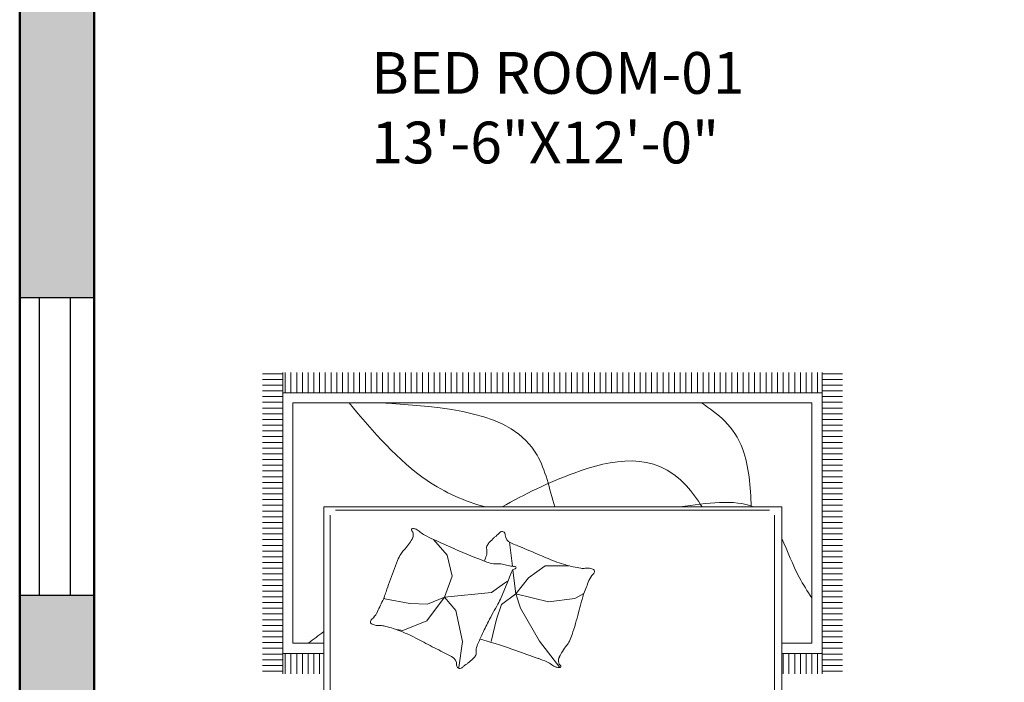
# Model space of a CAD drawing. Units: inches. Extents: x -7 to 1228, y -146 to 1091.
# Tile 4 of 88: x 60 to 179, y 112 to 193. Entities that reach past the tile are written whole.
import ezdxf

# ---------------------------------------------------------------- set-up
doc = ezdxf.new("R2010")
doc.units = ezdxf.units.IN
for name, color, linetype, lineweight in [('A-AREA-IDEN', 7, 'Continuous', 18), ('A-FURN', 8, 'Continuous', 18), ('A-GLAZ', 175, 'Continuous', 25), ('A-WALL', 7, 'Continuous', 50), ('A-WALL-PATT', 251, 'Continuous', 13)]:
    doc.layers.add(name, color=color, linetype=linetype, lineweight=lineweight)
doc.styles.add('DIM_FONT', font='SIMPLEX.shx', dxfattribs={"width": 0.8})
doc.styles.get("Standard").update_dxf_attribs({"font": 'arial.ttf'})

# ---------------------------------------------------------------- blocks, each defined once
blk = doc.blocks.new('A$C4F634EDD')
for p, q in [((0.5, 0.5295), (0.5, 2.6295)), ((2.3, 2.6295), (2.3, 0.5295)), ((0.5258, 2.121), (0.5258, 0.5617)), ((2.2716, 0.5617), (2.2716, 1.7136)), ((0.2586, 1.1753), (0.3386, 1.1753)), ((0.3386, 0), (0.3386, 1.1852)), ((0.3486, 1.1052), (0.3486, 1.1852)), ((0.3711, 1.1052), (0.3711, 1.1852)), ((0.3936, 1.1052), (0.3936, 1.1852)), ((0.4161, 1.1052), (0.4161, 1.1852)), ((0.4386, 1.1052), (0.4386, 1.1852)), ((0.4611, 1.1052), (0.4611, 1.1852)), ((0.4836, 1.1052), (0.4836, 1.1852)), ((1.031, 1.1612), (1.0448, 1.0581)), ((2.3061, 1.1052), (2.3061, 1.1852)), ((2.3286, 1.1052), (2.3286, 1.1852)), ((2.3511, 1.1052), (2.3511, 1.1852)), ((2.3736, 1.1052), (2.3736, 1.1852)), ((2.3961, 1.1052), (2.3961, 1.1852)), ((2.4186, 1.1052), (2.4186, 1.1852)), ((2.4411, 1.1052), (2.4411, 1.1852)), ((2.4588, 1.1852), (2.4588, 0)), ((2.4588, 1.1753), (2.5388, 1.1753)), ((0.2586, 1.1528), (0.3386, 1.1528)), ((0.2586, 1.1303), (0.3386, 1.1303)), ((1.4276, 1.1611), (1.3484, 1.0571)), ((2.4588, 1.1528), (2.5388, 1.1528)), ((2.4588, 1.1303), (2.5388, 1.1303)), ((0.2586, 1.1078), (0.3386, 1.1078)), ((0.2586, 1.0853), (0.3386, 1.0853)), ((0.3386, 1.1052), (0.5, 1.1052)), ((2.3, 1.1052), (2.4588, 1.1052)), ((2.4588, 1.1078), (2.5388, 1.1078)), ((2.4588, 1.0853), (2.5388, 1.0853)), ((0.2586, 1.0628), (0.3386, 1.0628)), ((0.3786, 1.0652), (0.5, 1.0652)), ((0.3786, 0.12), (0.3786, 1.0652)), ((1.0448, 1.0581), (1.019, 0.936)), ((1.1784, 0.9702), (1.1586, 1.0591)), ((1.3484, 1.0571), (1.2733, 0.9268)), ((2.3, 1.0652), (2.4188, 1.0652)), ((2.4188, 1.0652), (2.4188, 0.12)), ((2.4588, 1.0628), (2.5388, 1.0628)), ((0.2586, 1.0403), (0.3386, 1.0403)), ((0.2586, 1.0178), (0.3386, 1.0178)), ((0.8108, 1.0151), (0.7868, 1.0117)), ((0.9054, 0.9773), (0.8108, 1.0151)), ((2.4588, 1.0403), (2.5388, 1.0403)), ((2.4588, 1.0178), (2.5388, 1.0178)), ((0.2586, 0.9953), (0.3386, 0.9953)), ((0.2586, 0.9728), (0.3386, 0.9728)), ((0.9743, 0.8845), (0.9054, 0.9773)), ((1.1982, 0.9129), (1.1784, 0.9702)), ((2.4588, 0.9953), (2.5388, 0.9953)), ((2.4588, 0.9728), (2.5388, 0.9728)), ((0.2586, 0.9503), (0.3386, 0.9503)), ((1.019, 0.936), (0.9743, 0.8845)), ((2.4588, 0.9503), (2.5388, 0.9503)), ((0.2586, 0.9278), (0.3386, 0.9278)), ((0.2586, 0.9053), (0.3386, 0.9053)), ((0.7403, 0.8913), (0.737, 0.8849)), ((0.8384, 0.9085), (0.7403, 0.8913)), ((0.9072, 0.912), (0.8384, 0.9085)), ((0.9743, 0.8845), (0.9072, 0.912)), ((1.2555, 0.8715), (1.1982, 0.9129)), ((1.2733, 0.9268), (1.2555, 0.8715)), ((1.2555, 0.8715), (1.384, 0.9031)), ((1.384, 0.9031), (1.4868, 0.8892)), ((2.4588, 0.9278), (2.5388, 0.9278)), ((2.4588, 0.9053), (2.5388, 0.9053)), ((0.2586, 0.8828), (0.3386, 0.8828)), ((0.2586, 0.8603), (0.3386, 0.8603)), ((0.9743, 0.8845), (1.0052, 0.802)), ((0.9743, 0.8845), (1.16, 0.8656)), ((1.16, 0.8656), (1.2099, 0.8295)), ((1.1973, 0.8853), (1.2203, 0.829)), ((1.2555, 0.8715), (1.2437, 0.7773)), ((1.2555, 0.8715), (1.3049, 0.8082)), ((1.4868, 0.8892), (1.5228, 0.8692)), ((2.4588, 0.8828), (2.5388, 0.8828)), ((2.4588, 0.8603), (2.5388, 0.8603)), ((0.2586, 0.8378), (0.3386, 0.8378)), ((0.2586, 0.8153), (0.3386, 0.8153)), ((1.2099, 0.8295), (1.222, 0.8209)), ((1.2203, 0.829), (1.2381, 0.7855)), ((2.4588, 0.8378), (2.5388, 0.8378)), ((2.4588, 0.8153), (2.5388, 0.8153)), ((0.2586, 0.7928), (0.3386, 0.7928)), ((1.0052, 0.802), (0.9846, 0.7194)), ((1.3049, 0.8082), (1.3701, 0.7608)), ((2.4588, 0.7928), (2.5388, 0.7928)), ((0.2586, 0.7703), (0.3386, 0.7703)), ((0.2586, 0.7478), (0.3386, 0.7478)), ((1.2419, 0.7626), (1.23, 0.668)), ((1.3701, 0.7608), (1.463, 0.7608)), ((2.4588, 0.7703), (2.5388, 0.7703)), ((2.4588, 0.7478), (2.5388, 0.7478)), ((0.2586, 0.7253), (0.3386, 0.7253)), ((0.2586, 0.7028), (0.3386, 0.7028)), ((0.9846, 0.7194), (0.931, 0.6569)), ((2.4588, 0.7253), (2.5388, 0.7253)), ((2.4588, 0.7028), (2.5388, 0.7028)), ((0.2586, 0.6803), (0.3386, 0.6803)), ((2.4588, 0.6803), (2.5388, 0.6803)), ((0.2586, 0.6578), (0.3386, 0.6578)), ((0.2586, 0.6353), (0.3386, 0.6353)), ((2.4588, 0.6578), (2.5388, 0.6578)), ((2.4588, 0.6353), (2.5388, 0.6353)), ((0.2586, 0.6128), (0.3386, 0.6128)), ((0.2586, 0.5903), (0.3386, 0.5903)), ((2.4588, 0.6128), (2.5388, 0.6128)), ((2.4588, 0.5903), (2.5388, 0.5903)), ((0.2586, 0.5678), (0.3386, 0.5678)), ((0.2586, 0.5453), (0.3386, 0.5453)), ((2.4588, 0.5678), (2.5388, 0.5678)), ((2.4588, 0.5453), (2.5388, 0.5453)), ((0.2586, 0.5228), (0.3386, 0.5228)), ((2.3, 0.5295), (0.5, 0.5295)), ((0.5458, 0.5417), (2.2516, 0.5417)), ((2.4588, 0.5228), (2.5388, 0.5228)), ((0.2586, 0.5003), (0.3386, 0.5003)), ((0.2586, 0.4778), (0.3386, 0.4778)), ((2.4588, 0.5003), (2.5388, 0.5003)), ((2.4588, 0.4778), (2.5388, 0.4778)), ((0.2586, 0.4553), (0.3386, 0.4553)), ((0.2586, 0.4328), (0.3386, 0.4328)), ((2.4588, 0.4553), (2.5388, 0.4553)), ((2.4588, 0.4328), (2.5388, 0.4328)), ((0.2586, 0.4103), (0.3386, 0.4103)), ((0.2586, 0.3878), (0.3386, 0.3878)), ((2.4588, 0.4103), (2.5388, 0.4103)), ((2.4588, 0.3878), (2.5388, 0.3878)), ((0.2586, 0.3653), (0.3386, 0.3653)), ((2.4588, 0.3653), (2.5388, 0.3653)), ((0.2586, 0.3428), (0.3386, 0.3428)), ((0.2586, 0.3203), (0.3386, 0.3203)), ((2.4588, 0.3428), (2.5388, 0.3428)), ((2.4588, 0.3203), (2.5388, 0.3203)), ((0.2586, 0.2978), (0.3386, 0.2978)), ((0.2586, 0.2753), (0.3386, 0.2753)), ((2.4588, 0.2978), (2.5388, 0.2978)), ((2.4588, 0.2753), (2.5388, 0.2753)), ((0.2586, 0.2528), (0.3386, 0.2528)), ((2.4588, 0.2528), (2.5388, 0.2528)), ((0.2586, 0.2303), (0.3386, 0.2303)), ((0.2586, 0.2078), (0.3386, 0.2078)), ((2.4588, 0.2303), (2.5388, 0.2303)), ((2.4588, 0.2078), (2.5388, 0.2078)), ((0.2586, 0.1853), (0.3386, 0.1853)), ((0.2586, 0.1628), (0.3386, 0.1628)), ((2.4588, 0.1853), (2.5388, 0.1853)), ((2.4588, 0.1628), (2.5388, 0.1628)), ((0.2586, 0.1403), (0.3386, 0.1403)), ((0.2586, 0.1178), (0.3386, 0.1178)), ((2.4188, 0.12), (0.3786, 0.12)), ((2.4588, 0.1403), (2.5388, 0.1403)), ((2.4588, 0.1178), (2.5388, 0.1178)), ((0.2586, 0.0953), (0.3386, 0.0953)), ((2.4588, 0.08), (0.3386, 0.08)), ((0.3486, 0), (0.3486, 0.08)), ((0.3711, 0), (0.3711, 0.08)), ((0.3936, 0), (0.3936, 0.08)), ((0.4161, 0), (0.4161, 0.08)), ((0.4386, 0), (0.4386, 0.08)), ((0.4611, 0), (0.4611, 0.08)), ((0.4836, 0), (0.4836, 0.08)), ((0.5061, 0), (0.5061, 0.08)), ((0.5286, 0), (0.5286, 0.08)), ((0.5511, 0), (0.5511, 0.08)), ((0.5736, 0), (0.5736, 0.08)), ((0.5961, 0), (0.5961, 0.08)), ((0.6186, 0), (0.6186, 0.08)), ((0.6411, 0), (0.6411, 0.08)), ((0.6636, 0), (0.6636, 0.08)), ((0.6861, 0), (0.6861, 0.08)), ((0.7086, 0), (0.7086, 0.08)), ((0.7311, 0), (0.7311, 0.08)), ((0.7536, 0), (0.7536, 0.08)), ((0.7761, 0), (0.7761, 0.08)), ((0.7986, 0), (0.7986, 0.08)), ((0.8211, 0), (0.8211, 0.08)), ((0.8436, 0), (0.8436, 0.08)), ((0.8661, 0), (0.8661, 0.08)), ((0.8886, 0), (0.8886, 0.08)), ((0.9111, 0), (0.9111, 0.08)), ((0.9336, 0), (0.9336, 0.08)), ((0.9561, 0), (0.9561, 0.08)), ((0.9786, 0), (0.9786, 0.08)), ((1.0011, 0), (1.0011, 0.08)), ((1.0236, 0), (1.0236, 0.08)), ((1.0461, 0), (1.0461, 0.08)), ((1.0686, 0), (1.0686, 0.08)), ((1.0911, 0), (1.0911, 0.08)), ((1.1136, 0), (1.1136, 0.08)), ((1.1361, 0), (1.1361, 0.08)), ((1.1586, 0), (1.1586, 0.08)), ((1.1811, 0), (1.1811, 0.08)), ((1.2036, 0), (1.2036, 0.08)), ((1.2261, 0), (1.2261, 0.08)), ((1.2486, 0), (1.2486, 0.08)), ((1.2711, 0), (1.2711, 0.08)), ((1.2936, 0), (1.2936, 0.08)), ((1.3161, 0), (1.3161, 0.08)), ((1.3386, 0), (1.3386, 0.08)), ((1.3611, 0), (1.3611, 0.08)), ((1.3836, 0), (1.3836, 0.08)), ((1.4061, 0), (1.4061, 0.08)), ((1.4286, 0), (1.4286, 0.08)), ((1.4511, 0), (1.4511, 0.08)), ((1.4736, 0), (1.4736, 0.08)), ((1.4961, 0), (1.4961, 0.08)), ((1.5186, 0), (1.5186, 0.08)), ((1.5411, 0), (1.5411, 0.08)), ((1.5636, 0), (1.5636, 0.08)), ((1.5861, 0), (1.5861, 0.08)), ((1.6086, 0), (1.6086, 0.08)), ((1.6311, 0), (1.6311, 0.08)), ((1.6536, 0), (1.6536, 0.08)), ((1.6761, 0), (1.6761, 0.08)), ((1.6986, 0), (1.6986, 0.08)), ((1.7211, 0), (1.7211, 0.08)), ((1.7436, 0), (1.7436, 0.08)), ((1.7661, 0), (1.7661, 0.08)), ((1.7886, 0), (1.7886, 0.08)), ((1.8111, 0), (1.8111, 0.08)), ((1.8336, 0), (1.8336, 0.08)), ((1.8561, 0), (1.8561, 0.08)), ((1.8786, 0), (1.8786, 0.08)), ((1.9011, 0), (1.9011, 0.08)), ((1.9236, 0), (1.9236, 0.08)), ((1.9461, 0), (1.9461, 0.08)), ((1.9686, 0), (1.9686, 0.08)), ((1.9911, 0), (1.9911, 0.08)), ((2.0136, 0), (2.0136, 0.08)), ((2.0361, 0), (2.0361, 0.08)), ((2.0586, 0), (2.0586, 0.08)), ((2.0811, 0), (2.0811, 0.08)), ((2.1036, 0), (2.1036, 0.08)), ((2.1261, 0), (2.1261, 0.08)), ((2.1486, 0), (2.1486, 0.08)), ((2.1711, 0), (2.1711, 0.08)), ((2.1936, 0), (2.1936, 0.08)), ((2.2161, 0), (2.2161, 0.08)), ((2.2386, 0), (2.2386, 0.08)), ((2.2611, 0), (2.2611, 0.08)), ((2.2836, 0), (2.2836, 0.08)), ((2.3061, 0), (2.3061, 0.08)), ((2.3286, 0), (2.3286, 0.08)), ((2.3511, 0), (2.3511, 0.08)), ((2.3736, 0), (2.3736, 0.08)), ((2.3961, 0), (2.3961, 0.08)), ((2.4186, 0), (2.4186, 0.08)), ((2.4411, 0), (2.4411, 0.08)), ((2.4588, 0.0953), (2.5388, 0.0953)), ((0.2586, 0.0728), (0.3386, 0.0728)), ((0.2586, 0.0503), (0.3386, 0.0503)), ((2.4588, 0.0728), (2.5388, 0.0728)), ((2.4588, 0.0503), (2.5388, 0.0503)), ((0.2586, 0.0278), (0.3386, 0.0278)), ((0.2586, 0.0053), (0.3386, 0.0053)), ((2.4588, 0.0278), (2.5388, 0.0278)), ((2.4588, 0.0053), (2.5388, 0.0053))]:
    blk.add_line(p, q)
for centre, radius, start, end in [((1.0348, 1.1521), 0.0127, 51.1864, 183.2455), ((0.9991, 1.1077), 0.0697, 45.8726, 51.1864), ((1.4251, 1.1259), 0.0352, 86.0516, 110.3452), ((0.9863, 1.1494), 0.0359, 297.2902, 3.2455), ((1.0791, 1.1902), 0.0452, 225.8726, 232.4713), ((1.2846, 1.4577), 0.3825, 232.4713, 233.7837), ((0.6683, 0.6162), 0.6605, 52.7849, 53.7837), ((0.9362, 0.9689), 0.2176, 46.4776, 52.7849), ((1.0327, 1.0706), 0.0774, 35.8936, 46.4776), ((-0.4107, 5.9078), 5.0942, 289.0836, 290.1287), ((1.0543, 1.9106), 0.8371, 290.1287, 292.7069), ((1.3469, 1.2115), 0.0792, 292.7069, 308.5854), ((1.4338, 1.1026), 0.0601, 110.3452, 128.5854), ((1.4996, 1.1284), 0.0771, 169.5926, 177.2714), ((1.4378, 1.1314), 0.0153, 177.2714, 194.5709), ((1.4611, 1.1374), 0.0393, 194.5709, 206.8179), ((1.4376, 1.1398), 0.0142, 126.5792, 169.5926), ((1.4273, 1.1567), 0.00443, 13.2808, 86.0516), ((1.4254, 1.1562), 0.0063, 306.5792, 13.2808), ((1.8575, -0.7096), 2.0162, 116.4147, 117.4999), ((-0.4173, 3.8699), 3.0972, 296.4147, 297.2902), ((1.0771, 1.1027), 0.0226, 351.9508, 35.8936), ((1.1449, 1.0931), 0.0458, 171.9508, 202.4162), ((0.2266, 4.0657), 3.145, 286.6085, 289.0836), ((1.7401, 1.2785), 0.352, 206.8179, 210.9056), ((1.6045, 1.1973), 0.194, 210.9056, 219.7005), ((-1.8336, 6.2238), 5.8383, 297.49208, 297.84822), ((3.744, -4.3336), 6.1019, 117.49986, 117.84822), ((2.032, 1.4591), 1.0054, 202.4162, 205.0529), ((1.0922, 1.1636), 0.1166, 280.7366, 286.6085), ((1.3929, 1.0217), 0.081, 26.0735, 39.7005), ((1.2892, 0.9709), 0.1965, 17.8396, 26.0735), ((0.6422, 1.4168), 0.43, 282.6252, 290.7486), ((0.5736, 1.5979), 0.6236, 290.7486, 297.4921), ((2.6493, 1.7476), 1.6868, 205.0529, 207.0884), ((-0.4304, 0.4175), 2.003, 15.2625, 17.8396), ((0.6894, 0.9832), 0.0058, 121.6917, 179.0386), ((0.7004, 0.983), 0.0168, 179.0386, 229.4914), ((0.7131, 0.9448), 0.0509, 103.0402, 121.6917), ((0.6405, 0.9128), 0.0755, 26.3332, 49.4914), ((0.7152, 0.9361), 0.0599, 86.6119, 103.0402), ((0.7224, 1.0587), 0.063, 266.6119, 282.6252), ((2.541, 1.6922), 1.5652, 207.0884, 209.936), ((-1.6775, -0.2344), 2.6619, 25.1732, 26.3332), ((-0.0881, 0.5109), 1.6481, 13.841, 15.2625), ((0.5689, 0.8213), 0.1798, 20.7081, 25.1732), ((0.9989, 0.8042), 0.2143, 22.2355, 29.936), ((2.0418, 1.0357), 0.5454, 193.841, 196.3122), ((0.2268, 0.692), 0.5454, 18.2369, 20.7081), ((2.3102, 1.3785), 1.6481, 198.2369, 199.6584), ((1.6908, 0.933), 0.1798, 196.3122, 200.7773), ((4.0115, 1.8135), 2.6619, 200.7773, 201.9373), ((2.6444, 1.4979), 2.003, 199.6584, 202.2355), ((1.6124, 0.8472), 0.0755, 201.9373, 225.0955), ((1.2594, 0.7942), 0.0231, 202.2355, 252.8133), ((1.5375, 0.8209), 0.0509, 278.6443, 297.2959), ((1.5473, 0.7819), 0.0168, 354.6428, 45.0955), ((1.5582, 0.7808), 0.0058, 297.2959, 354.6428), ((0.9722, 0.8143), 0.1965, 202.2355, 210.4694), ((2.2689, -2.1899), 3.145, 111.0043, 113.4795), ((0.1831, 0.4093), 1.0054, 18.0203, 19.3448), ((1.1834, 0.6373), 0.1166, 98.1216, 111.0043), ((1.1763, 0.687), 0.0663, 85.4882, 98.1216), ((1.1871, 0.8241), 0.0712, 265.4882, 277.6784), ((1.1727, 0.9313), 0.1794, 277.6784, 284.8807), ((1.2689, 0.569), 0.1955, 97.9822, 104.8807), ((1.2465, 0.729), 0.034, 85.7407, 97.9822), ((1.2497, 0.772), 0.0092, 265.7407, 289.3799), ((1.2512, 0.7678), 0.00467, 289.3799, 72.8133), ((1.6266, 0.159), 0.6236, 106.3527, 113.0962), ((1.5721, 0.3449), 0.43, 98.2293, 106.3527), ((1.5195, 0.708), 0.063, 82.216, 98.2293), ((1.5362, 0.8298), 0.0599, 262.216, 278.6443), ((0.8727, 0.7557), 0.081, 210.4694, 224.0964), ((0.6752, 0.5644), 0.194, 35.3015, 44.0964), ((1.0957, 0.7061), 0.0458, 347.5549, 18.0203), ((0.5234, 2.5582), 2.0162, 292.0188, 293.104), ((-1.0798, 6.3161), 6.1019, 293.10398, 293.45234), ((3.6722, -4.6377), 5.8383, 113.0962, 113.45234), ((0.5462, 0.4731), 0.352, 31.2138, 35.3015), ((3.0455, -3.9778), 5.0942, 113.4795, 114.5246), ((1.1625, 0.6914), 0.0226, 167.5549, 211.4977), ((1.2092, 0.72), 0.0774, 211.4977, 222.0817), ((1.3133, 0.814), 0.2176, 222.0817, 228.389), ((1.2495, 0.6379), 0.0359, 112.8944, 178.8496), ((2.4404, -2.1823), 3.0972, 112.0188, 112.8944), ((0.8506, 0.6191), 0.0063, 130.9751, 197.6767), ((0.8372, 0.6345), 0.0142, 310.9751, 353.9885), ((0.8136, 0.6351), 0.0393, 18.9668, 31.2138), ((0.8364, 0.6429), 0.0153, 1.6673, 18.9668), ((0.7746, 0.6411), 0.0771, 353.9885, 1.6673), ((0.8382, 0.6719), 0.0601, 294.7411, 312.9813), ((0.9332, 0.57), 0.0792, 117.1028, 132.9813), ((1.2784, -0.1047), 0.8371, 114.5246, 117.1028), ((1.6074, 1.1451), 0.6605, 228.389, 229.3878), ((0.9284, 0.3533), 0.3825, 48.0754, 49.3878), ((1.1538, 0.6043), 0.0452, 41.4767, 48.0754), ((1.2399, 0.6804), 0.0697, 221.4767, 226.7905), ((1.2009, 0.6389), 0.0127, 226.7905, 358.8496), ((0.8488, 0.6185), 0.00443, 197.6767, 270.4475), ((0.8486, 0.6493), 0.0352, 270.4475, 294.7411)]:
    blk.add_arc(centre, radius, start, end)
for points in [[(0.4393, 1.0652), (0.4595, 1.05), (0.4798, 1.0348), (0.5, 1.0195)], [(1.9003, 0.5295), (2.0065, 0.514), (2.1132, 0.4978), (2.1894, 0.5295)]]:
    blk.add_open_spline(points, degree=3)
for points, knots in [([(2.3, 0.6535), (2.3236, 0.7026), (2.3554, 0.7914), (2.4015, 0.8608), (2.4188, 0.8868)], [1893.525221, 1893.525221, 1893.525221, 1893.525221, 2051.902476, 2146.74457, 2146.74457, 2146.74457, 2146.74457]), ([(0.5992, 0.12), (0.6957, 0.2341), (0.8523, 0.4189), (1.0536, 0.5069), (1.136, 0.5295)], [0, 0, 0, 0, 432.822832, 701.445452, 701.445452, 701.445452, 701.445452]), ([(0.7187, 0.12), (0.9791, 0.1362), (1.326, 0.1577), (1.3868, 0.4574), (1.408, 0.5295)], [0, 0, 0, 0, 653.160442, 870.050857, 870.050857, 870.050857, 870.050857]), ([(1.2016, 0.5295), (1.2892, 0.479), (1.5144, 0.3684), (1.8265, 0.2994), (1.9681, 0.4992), (1.9875, 0.5295)], [936.534237, 936.534237, 936.534237, 936.534237, 1243.285375, 1683.261222, 1758.254386, 1758.254386, 1758.254386, 1758.254386]), ([(2.1796, 0.5295), (2.1798, 0.4519), (2.1548, 0.2369), (2.0487, 0.164), (1.9846, 0.12)], [2202.034493, 2202.034493, 2202.034493, 2202.034493, 2357.807635, 2594.446174, 2594.446174, 2594.446174, 2594.446174])]:
    blk.add_open_spline(points, degree=3, knots=knots)
at = {"style": 'DIM_FONT', "width": 0.8, "flags": 9}
for tag, p in [('YSIZE', (0.5, 2.6295)), ('XSIZE', (0.5, 2.6295)), ('XSIZE', (2.2985, 2.6295)), ('YSIZE', (2.2985, 2.6295))]:
    blk.add_attdef(tag, p, '', height=0.0005, dxfattribs=at)
blk = doc.blocks.new('WIN-36')
for p, q in [((0, 36), (0, 0)), ((9, 36), (0, 36)), ((2.34, 36), (2.34, 0)), ((6.14, 0), (6.14, 36)), ((9, 0), (9, 36)), ((0, 0), (9, 0)), ((2.34, 0), (6.14, 0))]:
    blk.add_line(p, q)

msp = doc.modelspace()

# ---------------------------------------------------------------- hatches: boundary and pattern name
at = {"layer": 'A-WALL-PATT'}
h = msp.add_hatch(color=256, dxfattribs=at)
h.dxf.hatch_style = 1
h.paths.add_polyline_path([(69, 568), (60, 568), (60, 493), (63.29, 493), (69, 493)])
h.paths.add_polyline_path([(69, 662.41), (60, 662.41), (60, 586), (69, 586)], flags=17)
h.paths.add_polyline_path([(69, 723), (184, 723), (184, 734), (179, 734), (179, 728), (69, 728), (69, 741.62), (60, 741.62), (60, 698.41), (69, 698.41)], flags=17)
h.paths.add_polyline_path([(69, 782), (231, 782), (231, 728), (231, 723), (231, 586), (236, 586), (236, 787), (69, 787), (69, 800.13), (60, 800.13), (60, 765.62), (69, 765.62)])
h.paths.add_polyline_path([(184, 842), (189, 842), (189, 848), (173, 848), (173, 842), (179, 842), (179, 787), (184, 787)])
h.paths.add_polyline_path([(118.22, 69), (69, 69), (69, 60), (118.22, 60)])
h.paths.add_polyline_path([(227, 69), (154.22, 69), (154.22, 60), (227, 60)])
h.paths.add_polyline_path([(236, 60), (232.71, 60), (227, 60), (227, 36), (236, 36)])
h.paths.add_polyline_path([(389, 60), (380, 60), (380, 36), (389, 36)])
h.paths.add_polyline_path([(384, 181), (380, 181), (380, 115), (380, 78), (384, 78)])
h.paths.add_polyline_path([(380, 115), (334.55, 115), (334.55, 109), (380, 109)])
h.paths.add_polyline_path([(274.55, 115), (236, 115), (236, 201), (232.71, 201), (231, 201), (231, 78), (236, 78), (236, 109), (274.55, 109)])
h.paths.add_polyline_path([(69, 123), (60, 123), (60, 78), (69, 78)])
h.paths.add_polyline_path([(69, 201), (60, 201), (60, 159), (69, 159)])
h.paths.add_polyline_path([(143, 219), (69, 219), (69, 213), (143, 213)], flags=17)
h.paths.add_polyline_path([(189, 219), (184, 219), (184, 274), (231, 274), (231, 219), (236, 219), (236, 279), (184, 279), (184, 297), (179, 297), (179, 279), (69, 279), (69, 290.91), (60, 290.91), (60, 262.18), (69, 262.18), (69, 274), (179, 274), (179, 219), (173, 219), (173, 213), (189, 213)])
h.paths.add_polyline_path([(69, 238.18), (60, 238.18), (60, 219), (69, 219)], flags=17)
h.paths.add_polyline_path([(69, 333), (60, 333), (60, 314.91), (69, 314.91), (69, 316.96)])
h.paths.add_polyline_path([(190, 338), (184, 338), (69, 338), (69, 333), (179, 333), (179, 327), (184, 327), (184, 333.02), (190, 333.05)])
h.paths.add_polyline_path([(69, 386.81), (60, 386.81), (60, 351), (69, 351)])
h.paths.add_polyline_path([(69, 475), (60, 475), (60, 422.81), (69, 422.81)])
h.paths.add_polyline_path([(236, 475), (231, 475), (231, 351.24), (236, 351.24)])
h.paths.add_polyline_path([(384, 475), (380, 475), (380, 362), (384, 362)])
h.paths.add_polyline_path([(547, 307), (439, 307), (439, 356), (445, 356), (445, 362), (433, 362), (433, 307), (380, 307), (380, 244), (380, 241), (384, 241), (384, 301), (433, 301), (433, 277), (439, 277), (439, 301), (547, 301)])
h.paths.add_polyline_path([(547, 241), (439, 241), (439, 247), (433, 247), (433, 235), (547, 235)])
h.paths.add_polyline_path([(450, 69), (440.29, 69), (424.89, 69), (389, 69), (389, 60), (450, 60)])
h.paths.add_polyline_path([(547, 69), (486, 69), (486, 60), (547, 60)])
h.paths.add_polyline_path([(556, 148.27), (547, 148.27), (547, 78), (556, 78)])
h.paths.add_polyline_path([(556, 223), (547, 223), (547, 195), (547, 184.27), (556, 184.27)])
h.paths.add_polyline_path([(556, 311.19), (547, 311.19), (547, 273.08), (556, 273.08)])
h.paths.add_polyline_path([(556, 344), (552.71, 344), (547, 344), (547, 335.19), (556, 335.19)])
h.paths.add_polyline_path([(556, 249.08), (547, 249.08), (547, 241), (556, 241)])
h.paths.add_polyline_path([(547, 362), (475, 362), (475, 356), (547, 356)], flags=0)
h.paths.add_polyline_path([(556, 399.62), (547, 399.62), (547, 362), (556, 362)])
h.paths.add_polyline_path([(556, 475), (547, 475), (547, 435.62), (556, 435.62)])
h.paths.add_polyline_path([(547, 493), (389, 493), (389, 487), (547, 487)])
h.paths.add_polyline_path([(380, 493), (278, 493), (278, 487), (380, 487)])
h.paths.add_polyline_path([(227, 493), (69, 493), (69, 487), (227, 487)])
h.paths.add_polyline_path([(643, 122.44), (634, 122.44), (634, 78), (643, 78)])
h.paths.add_polyline_path([(702.5, 69), (692.79, 69), (677.39, 69), (643, 69), (643, 60), (702.5, 60)])
h.paths.add_polyline_path([(798, 69), (738.5, 69), (738.5, 60), (798, 60)])
h.paths.add_polyline_path([(807, 60), (803.71, 60), (798, 60), (798, 36), (807, 36)])
h.paths.add_polyline_path([(807, 109), (846.75, 109), (846.75, 115), (807, 115), (807, 159), (802, 159), (802, 78), (807, 78)])
h.paths.add_polyline_path([(807, 201), (802, 201), (802, 195), (807, 195)])
h.paths.add_polyline_path([(643, 201), (634, 201), (634, 158.44), (643, 158.44)])
h.paths.add_polyline_path([(756, 225), (751, 225), (751, 219), (643, 219), (643, 213), (756, 213)])
h.paths.add_polyline_path([(643, 240.85), (634, 240.85), (634, 219), (643, 219)])
h.paths.add_polyline_path([(643, 274), (643, 288.63), (634, 288.63), (634, 264.85), (643, 264.85)])
h.paths.add_polyline_path([(802, 279), (756, 279), (756, 297), (751, 297), (751, 279), (643, 279), (643, 274), (751, 274), (751, 255), (756, 255), (756, 274), (802, 274)])
h.paths.add_polyline_path([(807, 333), (803.71, 333), (802, 333), (802, 279), (802, 274), (802, 219), (807, 219)])
h.paths.add_polyline_path([(956, 182), (951, 182), (951, 115), (906.75, 115), (906.75, 109), (951, 109), (951, 78), (956, 78)])
h.paths.add_polyline_path([(960, 60), (951, 60), (951, 36), (960, 36)])
h.paths.add_polyline_path([(1021, 69), (1005.78, 69), (960, 69), (960, 60), (1021, 60)])
h.paths.add_polyline_path([(956, 224), (951, 224), (951, 218), (956, 218)])
h.paths.add_polyline_path([(956, 302), (1004, 302), (1004, 278), (1010, 278), (1010, 302), (1118, 302), (1118, 290.81), (1127, 290.81), (1127, 326.97), (1118, 326.97), (1118, 320.97), (1118, 307), (1010, 307), (1010, 356), (1016, 356), (1016, 362), (1004, 362), (1004, 307), (951, 307), (951, 244), (951, 242), (954.29, 242), (956, 242)])
h.paths.add_polyline_path([(643, 333), (634, 333), (634, 312.63), (643, 312.63), (643, 316.96)])
h.paths.add_polyline_path([(756, 338), (643, 338), (643, 333), (751, 333), (751, 327), (756, 327)])
h.paths.add_polyline_path([(643, 388), (634, 388), (634, 351), (643, 351)])
h.paths.add_polyline_path([(807, 357), (802, 357), (802, 351), (807, 351)])
h.paths.add_polyline_path([(807, 475), (802, 475), (802, 393), (807, 393)])
h.paths.add_polyline_path([(643, 475), (634, 475), (634, 424), (643, 424)])
h.paths.add_polyline_path([(798, 493), (643, 493), (643, 487), (798, 487)])
h.paths.add_polyline_path([(634, 493), (556, 493), (556, 487), (634, 487)])
h.paths.add_polyline_path([(813, 493), (807, 493), (807, 487), (813, 487)])
h.paths.add_polyline_path([(951, 493), (849, 493), (849, 487), (951, 487)])
h.paths.add_polyline_path([(956, 484), (951, 484), (951, 374), (956, 374)])
h.paths.add_polyline_path([(1109, 493), (969, 493), (969, 487), (1109, 487)])
h.paths.add_polyline_path([(1127, 484), (1118, 484), (1118, 450.64), (1127, 450.64)])
h.paths.add_polyline_path([(1127, 414.64), (1118, 414.64), (1118, 365), (1127, 365)])
h.paths.add_polyline_path([(1109, 362), (1046, 362), (1046, 356), (1109, 356)], flags=17)
h.paths.add_polyline_path([(1127, 356), (1123.45, 356), (1118, 356), (1118, 350.97), (1127, 350.97)], flags=0)
h.paths.add_polyline_path([(1127, 266.81), (1118, 266.81), (1118, 262.36), (1118, 242), (1127, 242)], flags=17)
h.paths.add_polyline_path([(1118, 242), (1010, 242), (1010, 248), (1004, 248), (1004, 237), (1118, 237)])
h.paths.add_polyline_path([(1127, 224), (1118, 224), (1118, 170), (1127, 170)])
h.paths.add_polyline_path([(1127, 134), (1118, 134), (1118, 78), (1127, 78)])
h.paths.add_polyline_path([(1118, 69), (1057, 69), (1057, 60), (1118, 60)])
h.paths.add_polyline_path([(227, 571.55), (227, 574), (69, 574), (69, 568), (227, 568)])
h.paths.add_polyline_path([(380, 571.55), (380, 574), (278, 574), (278, 568), (380, 568)])
h.paths.add_polyline_path([(242, 574), (236, 574), (236, 568), (242, 568)])
h.paths.add_polyline_path([(547, 571.55), (547, 574), (389, 574), (389, 568), (547, 568)])
h.paths.add_polyline_path([(384, 733), (380, 733), (380, 586), (384, 586)])
h.paths.add_polyline_path([(556, 646), (634, 646), (634, 655), (547, 655), (547, 586), (556, 586)])
h.paths.add_polyline_path([(634, 574), (556, 574), (556, 568), (634, 568)])
h.paths.add_polyline_path([(643, 655), (634, 655), (634, 586), (643, 586)])
h.paths.add_polyline_path([(798, 574), (643, 574), (643, 568), (798, 568)])
h.paths.add_polyline_path([(643, 663.85), (634, 663.85), (634, 655), (643, 655)])
h.paths.add_polyline_path([(556, 676.97), (547, 676.97), (547, 655), (556, 655)])
h.paths.add_polyline_path([(556, 733), (547, 733), (547, 712.97), (556, 712.97)])
h.paths.add_polyline_path([(643, 710), (634, 710), (634, 699.85), (643, 699.85)])
h.paths.add_polyline_path([(807, 668), (802, 668), (802, 586), (807, 586)])
h.paths.add_polyline_path([(951, 574), (849, 574), (849, 568), (951, 568)])
h.paths.add_polyline_path([(956, 691), (951, 691), (951, 577), (956, 577)])
h.paths.add_polyline_path([(1109, 574), (969, 574), (969, 568), (1109, 568)])
h.paths.add_polyline_path([(1127, 643.4), (1118, 643.4), (1118, 577), (1127, 577)])
h.paths.add_polyline_path([(1127, 568), (1123.45, 568), (1118, 568), (1118, 493), (1127, 493)])
h.paths.add_polyline_path([(1127, 733), (1118, 733), (1118, 679.4), (1127, 679.4)])
h.paths.add_polyline_path([(1127, 777.35), (1118, 777.35), (1118, 770.04), (1118, 751), (1127, 751)], flags=17)
h.paths.add_polyline_path([(1118, 751), (1010, 751), (1010, 757), (1004, 757), (1004, 745), (1118, 745)])
h.paths.add_polyline_path([(956, 811), (1004, 811), (1004, 787), (1010, 787), (1010, 811), (1017.87, 811), (1017.87, 811.63, -0.414214), (1018.25, 812), (1031.98, 812, -0.414214), (1032.35, 811.63), (1032.35, 811), (1118, 811), (1118, 801.35), (1127, 801.35), (1127, 834.69), (1118, 834.69), (1118, 830.24), (1118, 817), (1010, 817), (1010, 866), (1016, 866), (1016, 872), (1004, 872), (1004, 817), (956, 817), (956, 866), (951, 866), (951, 751), (954.29, 751), (956, 751)])
h.paths.add_polyline_path([(1118, 872), (1046, 872), (1046, 866), (1118, 866)], flags=17)
h.paths.add_polyline_path([(1127, 924.71), (1118, 924.71), (1118, 884), (1127, 884)])
h.paths.add_polyline_path([(1127, 866), (1123.71, 866), (1118, 866), (1118, 858.69), (1127, 858.69)], flags=17)
h.paths.add_polyline_path([(956, 983), (951, 983), (951, 952), (807, 952), (807, 983), (802, 983), (802, 902), (807, 902), (807, 946), (951, 946), (951, 884), (956, 884)])
h.paths.add_polyline_path([(807, 842), (802, 842), (802, 787), (756, 787), (756, 806), (751, 806), (751, 787), (643, 787), (643, 782), (751, 782), (751, 764), (756, 764), (756, 782), (802, 782), (802, 728), (807, 728)])
h.paths.add_polyline_path([(756, 848), (643, 848), (643, 842), (751, 842), (751, 836), (756, 836)])
h.paths.add_polyline_path([(756, 734), (751, 734), (751, 728), (643, 728), (643, 723), (756, 723)])
h.paths.add_polyline_path([(643, 749.79), (634, 749.79), (634, 728), (637.29, 728), (643, 728)])
h.paths.add_polyline_path([(643, 805.41), (634, 805.41), (634, 773.79), (643, 773.79)])
h.paths.add_polyline_path([(643, 896.66), (634, 896.66), (634, 860), (637.29, 860), (643, 860)])
h.paths.add_polyline_path([(643, 842), (634, 842), (634, 829.41), (643, 829.41)])
h.paths.add_polyline_path([(643, 983), (634, 983), (634, 932.66), (643, 932.66)])
h.paths.add_polyline_path([(1127, 983), (1118, 983), (1118, 960.71), (1127, 960.71)])
h.paths.add_polyline_path([(1118, 1001), (1077.53, 1001), (1077.53, 992), (1118, 992)])
h.paths.add_polyline_path([(1041.53, 1001), (960, 1001), (960, 992), (1041.53, 992)])
h.paths.add_polyline_path([(960, 1025), (951, 1025), (951, 1001), (954.29, 1001), (960, 1001)])
h.paths.add_polyline_path([(807, 1025), (798, 1025), (798, 1001), (807, 1001)])
h.paths.add_polyline_path([(798, 1001), (738.5, 1001), (738.5, 992), (798, 992)])
h.paths.add_polyline_path([(702.5, 1001), (643, 1001), (643, 992), (702.5, 992)])
h.paths.add_polyline_path([(547, 1001), (499.11, 1001), (499.11, 992), (547, 992)])
h.paths.add_polyline_path([(463.11, 1001), (389, 1001), (389, 992), (463.11, 992)])
h.paths.add_polyline_path([(389, 1025), (380, 1025), (380, 1022), (380, 1001), (383.29, 1001), (389, 1001)])
h.paths.add_polyline_path([(236, 1025), (227, 1025), (227, 1001), (236, 1001)])
h.paths.add_polyline_path([(236, 983), (231, 983), (231, 860), (236, 860)])
h.paths.add_polyline_path([(274.55, 952), (236, 952), (236, 946), (274.55, 946)])
h.paths.add_polyline_path([(380, 952), (334.55, 952), (334.55, 946), (380, 946)])
h.paths.add_polyline_path([(384, 983), (380, 983), (380, 884), (383.29, 884), (384, 884)])
h.paths.add_polyline_path([(227, 1001), (155.01, 1001), (155.01, 992), (162.87, 992), (227, 992)])
h.paths.add_polyline_path([(119.01, 1001), (69, 1001), (69, 992), (119.01, 992)])
h.paths.add_polyline_path([(69, 983), (60, 983), (60, 922.99), (69, 922.99)])
h.paths.add_polyline_path([(69, 886.99), (60, 886.99), (60, 860), (63.29, 860), (69, 860)])
h.paths.add_polyline_path([(143, 848), (69, 848), (69, 842), (143, 842)])

# ---------------------------------------------------------------- linework, layer by layer
at = {"layer": 'A-WALL'}
for p, q in [((60, 1001), (60, 60)), ((69, 274), (69, 60)), ((69, 69), (69, 213))]:
    msp.add_line(p, q, dxfattribs=at)

# ---------------------------------------------------------------- block references
at = {"layer": 'A-FURN', "xscale": -30.79356024027943, "yscale": 30.79356024027943, "zscale": 30.79356024027943, "rotation": 180}
msp.add_blockref('A$C4F634EDD', (81.41, 149.97), dxfattribs=at)
at = {"layer": 'A-GLAZ'}
msp.add_blockref('WIN-36', (60, 123), dxfattribs=at)

# ---------------------------------------------------------------- texts
at = {"layer": 'A-AREA-IDEN', "insert": (102.57, 188.76), "char_height": 5.0568, "attachment_point": 1}
msp.add_mtext_dynamic_manual_height_columns('BED ROOM-01\\P13\'-6"X12\'-0"', width=137.2821, gutter_width=25.28, heights=[0], dxfattribs=at)

doc.saveas('drawing.dxf')
